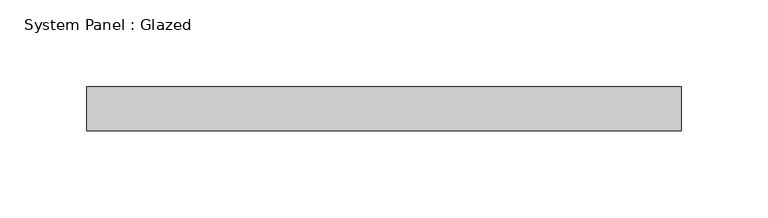
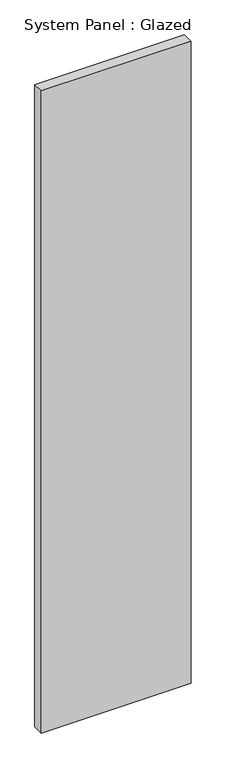
"""IFC4 building model written with IfcOpenShell, lengths in millimetres: plate geometry, System Panel : Glazed."""

from ifc_helpers import new_model, si_unit, origin, origin_with_axes, place, context, project, spatial, polyline, outline, extrude, source, transform, mapped, element, save


def system_panel_glazed_cd521809(model_context):
    return source(origin(), model_context, "Body", "SweptSolid", [
        extrude(outline(polyline([(171.45, 19.05), (-171.45, 19.05), (-171.45, 44.45), (171.45, 44.45), (171.45, 19.05)])), origin_with_axes(), (0.0, 0.0, 1.0), 1551.8095798),
    ])


if __name__ == "__main__":
    model = new_model("IFC4")
    model_context = context("Model", 3, world=origin())
    ifc_project = project(units=[si_unit("LENGTHUNIT", "METRE", prefix="MILLI")], contexts=[model_context])
    site = spatial("IfcSite", under=ifc_project)
    building = spatial("IfcBuilding", under=site)
    placement = place(None, origin())
    system_panel_glazed_shape = system_panel_glazed_cd521809(model_context)
    element("IfcPlate", 1, ObjectType="System Panel : Glazed", at=placement, inside=building, context=model_context, shape_type="MappedRepresentation", body=[
        mapped(system_panel_glazed_shape, transform((0.0, 0.0, 0.0), x_axis=(1.0, 0.0, 0.0), y_axis=(0.0, 1.0, 0.0), z_axis=(0.0, 0.0, 1.0))),
    ])
    save(model, "model.ifc")

# Revit data of these elements
# Type "System Panel : Glazed"
#   Construction Type Id = "GSP4R"
#   Analytic Construction = "1/8 in Pilkington single glazing"
#   Visual Light Transmittance = 0.9
#   Solar Heat Gain Coefficient = 0.86
#   Heat Transfer Coefficient (U) = 1.18115 BTU/(h·ft²·°F)
#   Define Thermal Properties by = 1
# Element 1 (IfcPlate, "System Panel : Glazed")
#   Materials on its faces: "Glass"
# Materials
#   "Glass": class "Glass", colour RGB 0 128 192, transparency 0.75, Description = "Soda Lime Glass", Cost = 0
